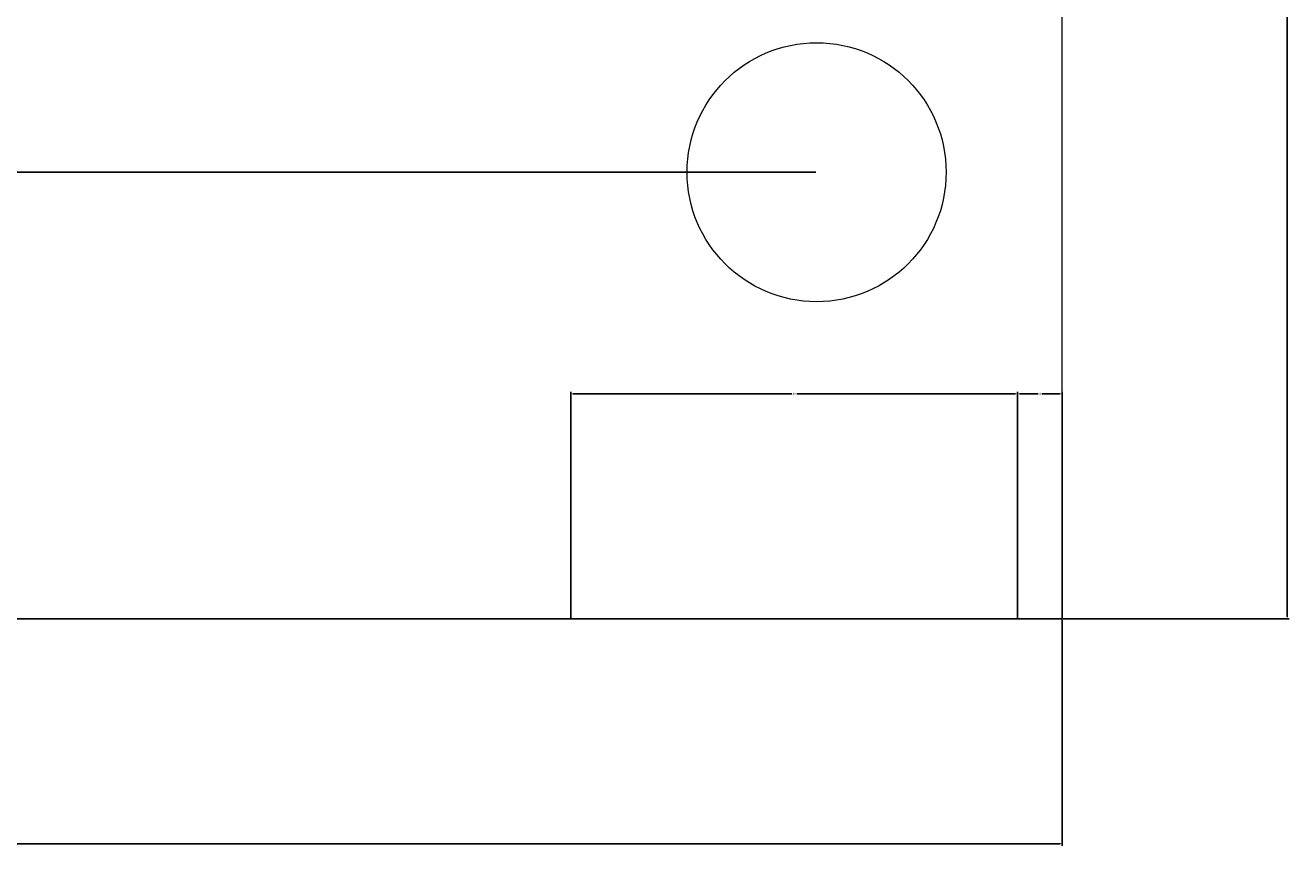
# Model space of a CAD drawing. Units: inches. Extents: x 1095 to 1408, y -20 to 240.
# Tile 6 of 8: x 1294 to 1408, y -20 to 53. Entities that reach past the tile are written whole.
import ezdxf

# ---------------------------------------------------------------- set-up
doc = ezdxf.new("R2010")
doc.units = ezdxf.units.IN
doc.header["$MEASUREMENT"] = 0
doc.layers.add('M-CONS', color=8, linetype='Continuous', lineweight=18)
doc.layers.add('M-DIMS', color=2, linetype='Continuous', lineweight=18)
doc.styles.get("Standard").update_dxf_attribs({"font": 'arial.ttf'})
doc.dimstyles.get("Standard").update_dxf_attribs({"dimtxt": 0.18, "dimasz": 0.18, "dimexe": 0.18, "dimexo": 0.0625, "dimgap": 0.09, "dimtad": 0, "dimtih": 1, "dimtoh": 1, "dimdec": 4, "dimzin": 0, "dimdsep": 46, "dimtxsty": 'Standard', "dimcen": 0.09, "dimadec": 0, "dimazin": 0, "dimtfac": 1, "dimtdec": 4, "dimtofl": 0, "dimtmove": 0, "dimatfit": 3, "dimfxl": 1, "dimtolj": 1, "dimtzin": 0, "dimarcsym": 0})

# ---------------------------------------------------------------- blocks, each defined once
blk = doc.blocks.new('*D1')
at = {"layer": 'Defpoints', "color": 0, "transparency": 16777216}
for p in [(1115.18, 0), (1387.18, 0), (1387.18, -20.15)]:
    blk.add_point(p, dxfattribs=at)
at = {"layer": 'M-DIMS', "color": 0, "lineweight": -2, "transparency": 16777216}
for p, q in [((1115.18, -0.06), (1115.18, -20.33)), ((1387.18, -0.06), (1387.18, -20.33)), ((1115.36, -20.15), (1250.89, -20.15)), ((1387, -20.15), (1251.47, -20.15))]:
    blk.add_line(p, q, dxfattribs=at)
at = {"layer": 'M-DIMS', "color": 0, "transparency": 16777216}
for points in [[(1115.36, -20.12), (1115.36, -20.18), (1115.18, -20.15)], [(1387, -20.12), (1387, -20.18), (1387.18, -20.15)]]:
    blk.add_solid(points, dxfattribs=at)
at = {"layer": 'M-DIMS', "color": 0, "transparency": 16777216, "insert": (1251.18, -20.15), "char_height": 0.18, "attachment_point": 5}
blk.add_mtext('\\A1;272', dxfattribs=at)
blk = doc.blocks.new('*D2')
at = {"layer": 'Defpoints', "color": 0, "transparency": 16777216}
for p in [(1365.18, 219.6), (1407.33, 219.6), (1387.18, 0)]:
    blk.add_point(p, dxfattribs=at)
at = {"layer": 'M-DIMS', "color": 0, "lineweight": -2, "transparency": 16777216}
for p, q in [((1365.25, 219.6), (1407.51, 219.6)), ((1407.33, 219.42), (1407.33, 109.98)), ((1407.33, 0.18), (1407.33, 109.62)), ((1387.25, 0), (1407.51, 0))]:
    blk.add_line(p, q, dxfattribs=at)
at = {"layer": 'M-DIMS', "color": 0, "transparency": 16777216}
for points in [[(1407.3, 219.42), (1407.36, 219.42), (1407.33, 219.6)], [(1407.3, 0.18), (1407.36, 0.18), (1407.33, 0)]]:
    blk.add_solid(points, dxfattribs=at)
at = {"layer": 'M-DIMS', "color": 0, "transparency": 16777216, "insert": (1407.33, 109.8), "char_height": 0.18, "attachment_point": 5}
blk.add_mtext('\\A1;219.6', dxfattribs=at)
blk = doc.blocks.new('*D8')
at = {"layer": 'Defpoints', "color": 0, "transparency": 16777216}
for p in [(1095.03, 124), (1387.18, 124), (1365.18, 40)]:
    blk.add_point(p, dxfattribs=at)
at = {"layer": 'M-DIMS', "color": 0, "lineweight": -2, "transparency": 16777216}
for p, q in [((1387.12, 124), (1094.85, 124)), ((1095.03, 123.82), (1095.03, 82.18)), ((1095.03, 40.18), (1095.03, 81.82)), ((1365.12, 40), (1094.85, 40))]:
    blk.add_line(p, q, dxfattribs=at)
at = {"layer": 'M-DIMS', "color": 0, "transparency": 16777216}
for points in [[(1095, 123.82), (1095.06, 123.82), (1095.03, 124)], [(1095, 40.18), (1095.06, 40.18), (1095.03, 40)]]:
    blk.add_solid(points, dxfattribs=at)
at = {"layer": 'M-DIMS', "color": 0, "transparency": 16777216, "insert": (1095.03, 82), "char_height": 0.18, "attachment_point": 5}
blk.add_mtext('\\A1;84', dxfattribs=at)
blk = doc.blocks.new('*D15')
at = {"layer": 'Defpoints', "color": 0, "transparency": 16777216}
for p in [(1383.18, 20.15), (1343.18, 0), (1383.18, 0)]:
    blk.add_point(p, dxfattribs=at)
at = {"layer": 'M-DIMS', "color": 0, "lineweight": -2, "transparency": 16777216}
for p, q in [((1343.18, 0.06), (1343.18, 20.33)), ((1343.36, 20.15), (1362.96, 20.15)), ((1383, 20.15), (1363.41, 20.15)), ((1383.18, 0.06), (1383.18, 20.33))]:
    blk.add_line(p, q, dxfattribs=at)
at = {"layer": 'M-DIMS', "color": 0, "transparency": 16777216}
for points in [[(1343.36, 20.18), (1343.36, 20.12), (1343.18, 20.15)], [(1383, 20.18), (1383, 20.12), (1383.18, 20.15)]]:
    blk.add_solid(points, dxfattribs=at)
at = {"layer": 'M-DIMS', "color": 0, "transparency": 16777216, "insert": (1363.18, 20.15), "char_height": 0.18, "attachment_point": 5}
blk.add_mtext('\\A1;40', dxfattribs=at)
blk = doc.blocks.new('*D16')
at = {"layer": 'Defpoints', "color": 0, "transparency": 16777216}
for p in [(1387.18, 20.15), (1383.18, 0), (1387.18, 0)]:
    blk.add_point(p, dxfattribs=at)
at = {"layer": 'M-DIMS', "color": 0, "lineweight": -2, "transparency": 16777216}
for p, q in [((1383.18, 0.06), (1383.18, 20.33)), ((1383.36, 20.15), (1385.03, 20.15)), ((1387, 20.15), (1385.34, 20.15)), ((1387.18, 0.06), (1387.18, 20.33))]:
    blk.add_line(p, q, dxfattribs=at)
at = {"layer": 'M-DIMS', "color": 0, "transparency": 16777216}
for points in [[(1383.36, 20.18), (1383.36, 20.12), (1383.18, 20.15)], [(1387, 20.18), (1387, 20.12), (1387.18, 20.15)]]:
    blk.add_solid(points, dxfattribs=at)
at = {"layer": 'M-DIMS', "color": 0, "transparency": 16777216, "insert": (1385.18, 20.15), "char_height": 0.18, "attachment_point": 5}
blk.add_mtext('\\A1;4', dxfattribs=at)

msp = doc.modelspace()

# ---------------------------------------------------------------- linework, layer by layer
at = {"layer": 'M-CONS', "extrusion": (0, -1, 0)}
for p, q in [((1387.184, 0, 397.783), (1387.184, 124, 397.783)), ((1115.184, 0, 357.783), (1387.184, 0, 357.783)), ((1383.184, 0, 377.783), (1119.184, 0, 377.783)), ((1387.184, 0, 397.783), (1343.184, 0, 397.783)), ((1343.184, 0, 397.783), (1343.184, 0, 392.783)), ((1343.184, 0, 392.783), (1383.184, 0, 392.783)), ((1383.184, 0, 392.783), (1383.184, 0, 377.783)), ((1387.184, 0, 357.783), (1387.184, 0, 397.783))]:
    msp.add_line(p, q, dxfattribs=at)
at = {"layer": 'M-CONS'}
msp.add_circle((1365.184, 40, 397.783), 11.6, dxfattribs=at)

# ---------------------------------------------------------------- dimensions: what is measured, and where the dimension line sits
at = {"layer": 'M-DIMS'}
for base, p1, p2, override, picture, middle in [((1407.334, 219.6), (1387.184, 0), (1365.184, 219.6), {"dimdec": 1, "dimlfac": 1, "dimrnd": 0, "dimzin": 0, "dimdsep": 46, "dimlunit": 2}, '*D2', (1407.334, 109.8)), ((1095.034, 124), (1365.184, 40), (1387.184, 124), {"dimdec": 0, "dimlfac": 1, "dimrnd": 0, "dimzin": 0, "dimdsep": 46, "dimlunit": 2}, '*D8', (1095.034, 82))]:
    dim = msp.add_linear_dim(base=base, p1=p1, p2=p2, angle=90, dimstyle='Standard', override=override, dxfattribs=at)
    dim.commit()
    dim.dimension.update_dxf_attribs({"geometry": picture, "text_midpoint": middle})
for base, p1, p2, picture, middle in [((1383.184, 20.15), (1343.184, 0), (1383.184, 0), '*D15', (1363.184, 20.15)), ((1387.184, 20.15), (1383.184, 0), (1387.184, 0), '*D16', (1385.184, 20.15)), ((1387.184, -20.15), (1115.184, 0), (1387.184, 0), '*D1', (1251.184, -20.15))]:
    dim = msp.add_linear_dim(base=base, p1=p1, p2=p2, dimstyle='Standard', override={"dimdec": 0, "dimlfac": 1, "dimrnd": 0, "dimzin": 0, "dimdsep": 46, "dimlunit": 2}, dxfattribs=at)
    dim.commit()
    dim.dimension.update_dxf_attribs({"geometry": picture, "text_midpoint": middle})

doc.saveas('drawing.dxf')
